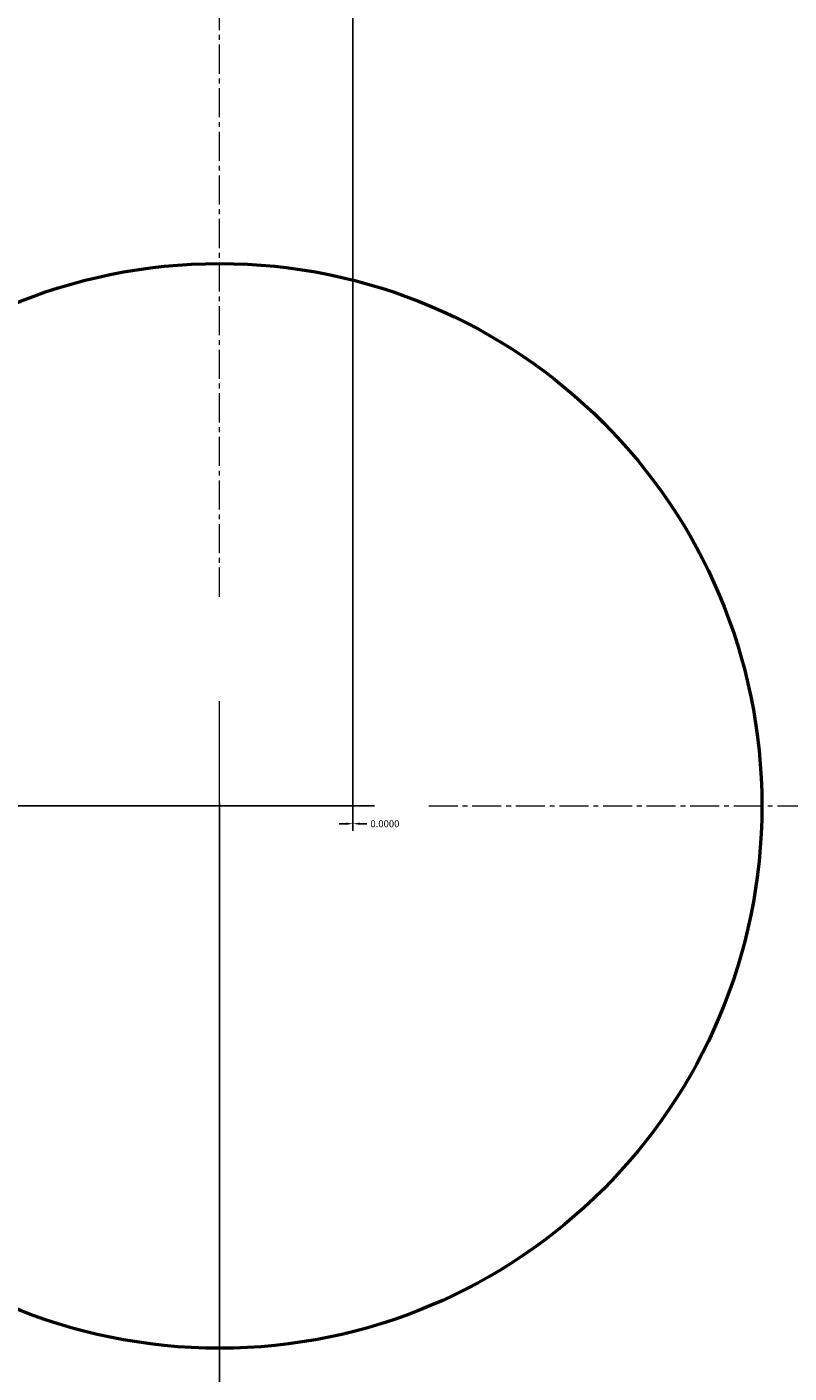
# Model space of a CAD drawing. Units: millimetres. Extents: x -60 to 113, y -37 to 126.
# Tile 4 of 17: x 2 to 22, y -8 to 27. Entities that reach past the tile are written whole.
import ezdxf

# ---------------------------------------------------------------- set-up
doc = ezdxf.new("R2010")
doc.units = ezdxf.units.MM
doc.header["$MEASUREMENT"] = 0
doc.linetypes.add('CENTER2', pattern=[1.125, 0.75, -0.125, 0.125, -0.125])
for name, color, linetype, lineweight in [('M-CNTR', 4, 'CENTER2', 18), ('M-DIMS', 2, 'Continuous', 25), ('M-OUTL', 7, 'Continuous', 50)]:
    doc.layers.add(name, color=color, linetype=linetype, lineweight=lineweight)
doc.styles.get("Standard").update_dxf_attribs({"font": 'arial.ttf'})
doc.dimstyles.get("Standard").update_dxf_attribs({"dimtxt": 0.18, "dimasz": 0.18, "dimexe": 0.18, "dimexo": 0.0625, "dimgap": 0.09, "dimtad": 0, "dimtih": 1, "dimtoh": 1, "dimdec": 4, "dimzin": 0, "dimdsep": 46, "dimtxsty": 'Standard', "dimcen": 0.09, "dimadec": 0, "dimazin": 0, "dimtfac": 1, "dimtdec": 4, "dimtofl": 0, "dimtmove": 0, "dimatfit": 3, "dimfxl": 1, "dimtolj": 1, "dimtzin": 0, "dimarcsym": 0})

# ---------------------------------------------------------------- blocks, each defined once
blk = doc.blocks.new('*U2')
at = {"layer": 'M-CNTR', "color": 0, "transparency": 16777216}
for p, q in [((0, 5.4), (0, 27.12)), ((5.4, 0), (27.12, 0)), ((0, -27.12), (0, -5.4))]:
    blk.add_line(p, q, dxfattribs=at)
at = {"layer": 'M-CNTR', "color": 0, "linetype": 'Continuous', "transparency": 16777216}
for p, q in [((0, -2.7), (0, 2.7)), ((-2.7, 0), (2.7, 0))]:
    blk.add_line(p, q, dxfattribs=at)
blk = doc.blocks.new('*D12')
at = {"layer": 'Defpoints', "color": 0, "transparency": 16777216}
for p in [(10.532, 88.533), (-58.719, 6.903), (11.329, 6.903)]:
    blk.add_point(p, dxfattribs=at)
at = {"layer": 'M-DIMS', "color": 0, "lineweight": -2, "transparency": 16777216}
for p, q in [((10.47, 88.533), (-58.899, 88.533)), ((-58.719, 88.353), (-58.719, 48.829)), ((-58.719, 7.083), (-58.719, 46.607)), ((11.267, 6.903), (-58.899, 6.903))]:
    blk.add_line(p, q, dxfattribs=at)
at = {"layer": 'M-DIMS', "color": 0, "transparency": 16777216}
for points in [[(-58.749, 88.353), (-58.689, 88.353), (-58.719, 88.533)], [(-58.749, 7.083), (-58.689, 7.083), (-58.719, 6.903)]]:
    blk.add_solid(points, dxfattribs=at)
at = {"layer": 'M-DIMS', "color": 0, "transparency": 16777216, "insert": (-58.719, 47.718), "char_height": 0.18, "attachment_point": 5}
blk.add_mtext('\\A1;{\\H11.11111x;82}', dxfattribs=at)
blk = doc.blocks.new('*D13')
at = {"layer": 'Defpoints', "color": 0, "transparency": 16777216}
for p in [(37.065, 46.813), (-39.303, 6.903), (7.267, 6.903)]:
    blk.add_point(p, dxfattribs=at)
at = {"layer": 'M-DIMS', "color": 0, "lineweight": -2, "transparency": 16777216}
for p, q in [((37.002, 46.813), (-39.483, 46.813)), ((-39.303, 46.633), (-39.303, 27.969)), ((-39.303, 7.083), (-39.303, 25.747)), ((7.204, 6.903), (-39.483, 6.903))]:
    blk.add_line(p, q, dxfattribs=at)
at = {"layer": 'M-DIMS', "color": 0, "transparency": 16777216}
for points in [[(-39.333, 46.633), (-39.273, 46.633), (-39.303, 46.813)], [(-39.333, 7.083), (-39.273, 7.083), (-39.303, 6.903)]]:
    blk.add_solid(points, dxfattribs=at)
at = {"layer": 'M-DIMS', "color": 0, "transparency": 16777216, "insert": (-39.303, 26.858), "char_height": 0.18, "attachment_point": 5}
blk.add_mtext('\\A1;{\\H11.11111x;40}', dxfattribs=at)
blk = doc.blocks.new('*D14')
at = {"layer": 'Defpoints', "color": 0, "transparency": 16777216}
for p in [(7.267, 6.903), (67.355, 6.442), (67.355, -36.011)]:
    blk.add_point(p, dxfattribs=at)
at = {"layer": 'M-DIMS', "color": 0, "lineweight": -2, "transparency": 16777216}
for p, q in [((7.267, 6.84), (7.267, -36.191)), ((67.355, 6.379), (67.355, -36.191)), ((7.447, -36.011), (35.786, -36.011)), ((67.175, -36.011), (38.835, -36.011))]:
    blk.add_line(p, q, dxfattribs=at)
at = {"layer": 'M-DIMS', "color": 0, "transparency": 16777216}
for points in [[(7.447, -35.981), (7.447, -36.041), (7.267, -36.011)], [(67.175, -35.981), (67.175, -36.041), (67.355, -36.011)]]:
    blk.add_solid(points, dxfattribs=at)
at = {"layer": 'M-DIMS', "color": 0, "transparency": 16777216, "insert": (37.311, -36.011), "char_height": 0.18, "attachment_point": 5}
blk.add_mtext('\\A1;{\\H11.11111x;60}', dxfattribs=at)
blk = doc.blocks.new('*D15')
at = {"layer": 'Defpoints', "color": 0, "transparency": 16777216}
for p in [(17.836, 16.083), (-3.303, -2.278)]:
    blk.add_point(p, dxfattribs=at)
at = {"layer": 'M-DIMS', "color": 0, "lineweight": -2, "transparency": 16777216}
for p, q in [((7.267, 6.813), (7.267, 6.993)), ((7.177, 6.903), (7.357, 6.903)), ((-20.464, -17.184), (-3.439, -2.396)), ((-20.644, -17.184), (-20.464, -17.184))]:
    blk.add_line(p, q, dxfattribs=at)
at = {"layer": 'M-DIMS', "color": 0, "transparency": 16777216}
blk.add_solid([(-3.459, -2.373), (-3.419, -2.419), (-3.303, -2.278)], dxfattribs=at)
at = {"layer": 'M-DIMS', "color": 0, "transparency": 16777216, "insert": (-24.497, -17.184), "char_height": 0.18, "attachment_point": 5}
blk.add_mtext('\\A1;{\\H11.11111x;3-%%C28}', dxfattribs=at)
blk = doc.blocks.new('*D16')
at = {"layer": 'Defpoints', "color": 0, "transparency": 16777216}
for p in [(10.712, 88.533), (10.712, 88.533), (10.712, 6.442)]:
    blk.add_point(p, dxfattribs=at)
at = {"layer": 'M-DIMS', "color": 0, "lineweight": -2, "transparency": 16777216}
for p, q in [((10.712, 88.47), (10.712, 6.262)), ((10.712, 88.47), (10.712, 6.262)), ((10.532, 6.442), (10.352, 6.442)), ((10.892, 6.442), (11.072, 6.442))]:
    blk.add_line(p, q, dxfattribs=at)
at = {"layer": 'M-DIMS', "color": 0, "transparency": 16777216}
for points in [[(10.532, 6.472), (10.532, 6.412), (10.712, 6.442)], [(10.892, 6.472), (10.892, 6.412), (10.712, 6.442)]]:
    blk.add_solid(points, dxfattribs=at)
at = {"layer": 'M-DIMS', "color": 0, "transparency": 16777216, "insert": (11.536, 6.442), "char_height": 0.18, "attachment_point": 5}
blk.add_mtext('\\A1;0.0000', dxfattribs=at)
blk = doc.blocks.new('*D17')
at = {"layer": 'Defpoints', "color": 0, "transparency": 16777216}
for p in [(67.355, 124.823), (10.532, 88.533), (67.355, 6.442)]:
    blk.add_point(p, dxfattribs=at)
at = {"layer": 'M-DIMS', "color": 0, "lineweight": -2, "transparency": 16777216}
for p, q in [((10.532, 88.595), (10.532, 125.003)), ((10.712, 124.823), (37.422, 124.823)), ((67.175, 124.823), (40.465, 124.823)), ((67.355, 6.504), (67.355, 125.003))]:
    blk.add_line(p, q, dxfattribs=at)
at = {"layer": 'M-DIMS', "color": 0, "transparency": 16777216}
for points in [[(10.712, 124.853), (10.712, 124.793), (10.532, 124.823)], [(67.175, 124.853), (67.175, 124.793), (67.355, 124.823)]]:
    blk.add_solid(points, dxfattribs=at)
at = {"layer": 'M-DIMS', "color": 0, "transparency": 16777216, "insert": (38.944, 124.823), "char_height": 0.18, "attachment_point": 5}
blk.add_mtext('\\A1;{\\H11.11111x;56}', dxfattribs=at)
blk = doc.blocks.new('HOLE-D28')
blk.add_circle((14, 14), 14)

msp = doc.modelspace()

# ---------------------------------------------------------------- linework, layer by layer
at = {"layer": 'M-OUTL'}
msp.add_arc((7.26659, 6.9027), 27, 131.866655, 323.73509, dxfattribs=at)

# ---------------------------------------------------------------- block references
at = {"layer": 'M-CNTR'}
msp.add_blockref('*U2', (7.26659, 6.9027), dxfattribs=at)
at = {"layer": 'M-OUTL'}
msp.add_blockref('HOLE-D28', (-6.733, -7.097), dxfattribs=at)

# ---------------------------------------------------------------- dimensions: what is measured, and where the dimension line sits
at = {"layer": 'M-DIMS'}
for base, p1, text, picture, middle in [((67.35481, 124.82251), (10.53227, 88.53289), '{\\H11.11111x;56}', '*D17', (38.94354, 124.82251)), ((67.35481, -36.0105), (7.26659, 6.9027), '{\\H11.11111x;60}', '*D14', (37.3107, -36.0105))]:
    dim = msp.add_linear_dim(base=base, p1=p1, p2=(67.35481, 6.44179), text=text, dimstyle='Standard', override={"dimclrd": 0, "dimclre": 0, "dimclrt": 0}, dxfattribs=at)
    dim.commit()
    dim.dimension.update_dxf_attribs({"geometry": picture, "text_midpoint": middle})
for base, p1, p2, text, picture, middle in [((-58.71857, 6.9027), (10.53227, 88.53289), (11.32938, 6.9027), '{\\H11.11111x;82}', '*D12', (-58.71857, 47.71779)), ((-39.30316, 6.9027), (37.06463, 46.81263), (7.26659, 6.9027), '{\\H11.11111x;40}', '*D13', (-39.30316, 26.85766))]:
    dim = msp.add_linear_dim(base=base, p1=p1, p2=p2, angle=90, text=text, dimstyle='Standard', override={"dimclrd": 0, "dimclre": 0, "dimclrt": 0}, dxfattribs=at)
    dim.commit()
    dim.dimension.update_dxf_attribs({"geometry": picture, "text_midpoint": middle})
dim = msp.add_linear_dim(base=(10.712269814, 6.441792179), p1=(10.712269814, 88.5328900903), p2=(10.712269814, 88.5328900903), dimstyle='Standard', override={"dimclrd": 0, "dimclre": 0, "dimclrt": 0}, dxfattribs=at)
dim.commit()
dim.dimension.update_dxf_attribs({"geometry": '*D16', "text_midpoint": (11.5355917785, 6.441792179)})
dim = msp.add_diameter_dim_2p(p1=(17.83613, 16.08337), p2=(-3.30296, -2.27798), text='{\\H11.11111x;3-%%C28}', dimstyle='Standard', override={"dimclrd": 0, "dimclre": 0, "dimclrt": 0}, dxfattribs=at)
dim.commit()
dim.dimension.update_dxf_attribs({"geometry": '*D15', "text_midpoint": (-24.49681, -17.18418), "dimtype": 163})

doc.saveas('drawing.dxf')
